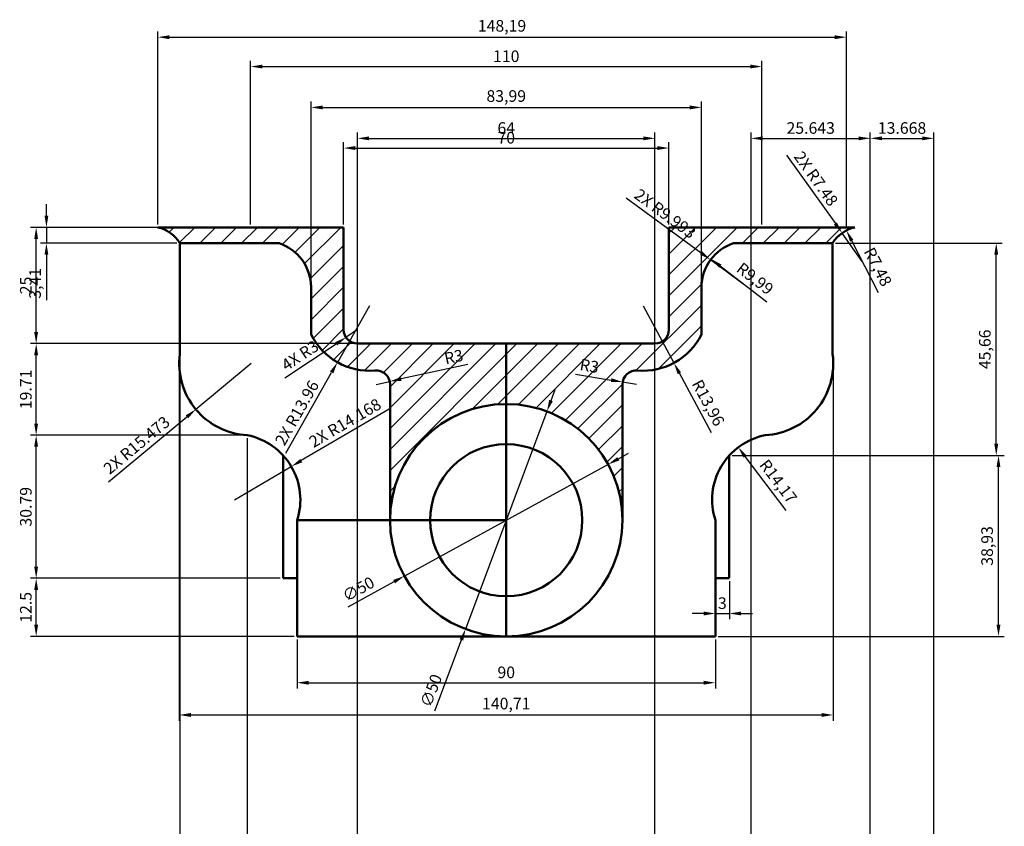
# Model space of a CAD drawing. Units: millimetres. Extents: x 2172 to 2566, y 897 to 1244.
# Tile 2 of 3: x 2172 to 2384, y 1071 to 1244. Entities that reach past the tile are written whole.
import ezdxf

# ---------------------------------------------------------------- set-up
doc = ezdxf.new("R2010")
doc.units = ezdxf.units.MM
for name, color, linetype, lineweight in [('M-DIMS', 2, 'Continuous', 25), ('M-HATC', 8, 'Continuous', 18), ('M-OUTL', 7, 'Continuous', 50)]:
    doc.layers.add(name, color=color, linetype=linetype, lineweight=lineweight)
doc.styles.get("Standard").update_dxf_attribs({"font": 'arial.ttf'})
doc.dimstyles.new('ISO-25', dxfattribs={"dimtxt": 2.5, "dimasz": 2.5, "dimexe": 1.25, "dimexo": 0.625, "dimtad": 1, "dimtxsty": 'Standard', "dimcen": 2.5, "dimadec": 0, "dimazin": 0, "dimtfac": 1, "dimtmove": 0, "dimatfit": 3, "dimfxl": 1, "dimarcsym": 0})

# ---------------------------------------------------------------- blocks, each defined once
blk = doc.blocks.new('*D19')
at = {"layer": 'Defpoints', "color": 0, "transparency": 16777216}
for p in [(2206.43, 1170.23), (2347.14, 1170.23), (2347.14, 1094.59)]:
    blk.add_point(p, dxfattribs=at)
at = {"layer": 'M-DIMS', "color": 0, "lineweight": -2, "transparency": 16777216}
for p, q in [((2206.43, 1169.6), (2206.43, 1093.34)), ((2347.14, 1169.6), (2347.14, 1093.34)), ((2208.93, 1094.59), (2344.64, 1094.59))]:
    blk.add_line(p, q, dxfattribs=at)
at = {"layer": 'M-DIMS', "color": 0, "transparency": 16777216}
for points in [[(2208.93, 1095.01), (2208.93, 1094.17), (2206.43, 1094.59)], [(2344.64, 1095.01), (2344.64, 1094.17), (2347.14, 1094.59)]]:
    blk.add_solid(points, dxfattribs=at)
at = {"layer": 'M-DIMS', "color": 0, "transparency": 16777216, "insert": (2276.79, 1096.72), "char_height": 2.5, "attachment_point": 5}
blk.add_mtext('140,71', dxfattribs=at)
blk = doc.blocks.new('*D20')
at = {"layer": 'Defpoints', "color": 0, "transparency": 16777216}
for p in [(2231.79, 1111.49), (2321.79, 1111.49), (2321.79, 1101.53)]:
    blk.add_point(p, dxfattribs=at)
at = {"layer": 'M-DIMS', "color": 0, "lineweight": -2, "transparency": 16777216}
for p, q in [((2231.79, 1110.86), (2231.79, 1100.28)), ((2321.79, 1110.86), (2321.79, 1100.28)), ((2234.29, 1101.53), (2319.29, 1101.53))]:
    blk.add_line(p, q, dxfattribs=at)
at = {"layer": 'M-DIMS', "color": 0, "transparency": 16777216}
for points in [[(2234.29, 1101.94), (2234.29, 1101.11), (2231.79, 1101.53)], [(2319.29, 1101.94), (2319.29, 1101.11), (2321.79, 1101.53)]]:
    blk.add_solid(points, dxfattribs=at)
at = {"layer": 'M-DIMS', "color": 0, "transparency": 16777216, "insert": (2276.79, 1103.43), "char_height": 2.5, "attachment_point": 5}
blk.add_mtext('90', dxfattribs=at)
blk = doc.blocks.new('*D21')
at = {"layer": 'Defpoints', "color": 0, "transparency": 16777216}
for p in [(2298.71, 1148.5), (2254.86, 1124.48)]:
    blk.add_point(p, dxfattribs=at)
at = {"layer": 'M-DIMS', "color": 0, "lineweight": -2, "transparency": 16777216}
for p, q in [((2300.91, 1149.7), (2303.1, 1150.9)), ((2298.71, 1148.5), (2254.86, 1124.48)), ((2242.77, 1117.85), (2252.67, 1123.27))]:
    blk.add_line(p, q, dxfattribs=at)
at = {"layer": 'M-DIMS', "color": 0, "transparency": 16777216}
for points in [[(2300.71, 1150.07), (2301.11, 1149.33), (2298.71, 1148.5)], [(2252.47, 1123.64), (2252.87, 1122.91), (2254.86, 1124.48)]]:
    blk.add_solid(points, dxfattribs=at)
at = {"layer": 'M-DIMS', "color": 0, "transparency": 16777216, "insert": (2245.13, 1121.39), "char_height": 2.5, "attachment_point": 5, "rotation": 28.7152}
blk.add_mtext('∅50', dxfattribs=at)
blk = doc.blocks.new('*D22')
at = {"layer": 'Defpoints', "color": 0, "transparency": 16777216}
for p in [(2326.7, 1152.17), (2335.26, 1140.88)]:
    blk.add_point(p, dxfattribs=at)
at = {"layer": 'M-DIMS', "color": 0, "lineweight": -2, "transparency": 16777216}
blk.add_line((2337.02, 1138.56), (2328.21, 1150.18), dxfattribs=at)
at = {"layer": 'M-DIMS', "color": 0, "transparency": 16777216}
blk.add_solid([(2328.54, 1150.43), (2327.88, 1149.92), (2326.7, 1152.17)], dxfattribs=at)
at = {"layer": 'M-DIMS', "color": 0, "transparency": 16777216, "insert": (2335.07, 1144.65), "char_height": 2.5, "attachment_point": 5, "rotation": 307.1523}
blk.add_mtext('R14,17', dxfattribs=at)
blk = doc.blocks.new('*D23')
at = {"layer": 'Defpoints', "color": 0, "transparency": 16777216}
for p in [(2306.24, 1182.6), (2312.86, 1170.31)]:
    blk.add_point(p, dxfattribs=at)
at = {"layer": 'M-DIMS', "color": 0, "lineweight": -2, "transparency": 16777216}
for p, q in [((2306.24, 1182.6), (2312.86, 1170.31)), ((2320.96, 1155.28), (2314.04, 1168.11))]:
    blk.add_line(p, q, dxfattribs=at)
at = {"layer": 'M-DIMS', "color": 0, "transparency": 16777216}
blk.add_solid([(2314.41, 1168.31), (2313.68, 1167.91), (2312.86, 1170.31)], dxfattribs=at)
at = {"layer": 'M-DIMS', "color": 0, "transparency": 16777216, "insert": (2319.97, 1161.6), "char_height": 2.5, "attachment_point": 5, "rotation": 298.3069}
blk.add_mtext('R13,96', dxfattribs=at)
blk = doc.blocks.new('*D24')
at = {"layer": 'Defpoints', "color": 0, "transparency": 16777216}
for p in [(2320.87, 1192.69), (2328.77, 1186.58)]:
    blk.add_point(p, dxfattribs=at)
at = {"layer": 'M-DIMS', "color": 0, "lineweight": -2, "transparency": 16777216}
blk.add_line((2332.85, 1183.43), (2322.85, 1191.16), dxfattribs=at)
at = {"layer": 'M-DIMS', "color": 0, "transparency": 16777216}
blk.add_solid([(2323.1, 1191.49), (2322.59, 1190.83), (2320.87, 1192.69)], dxfattribs=at)
at = {"layer": 'M-DIMS', "color": 0, "transparency": 16777216, "insert": (2330.14, 1188.21), "char_height": 2.5, "attachment_point": 5, "rotation": 322.2747}
blk.add_mtext('R9,99', dxfattribs=at)
blk = doc.blocks.new('*D25')
at = {"layer": 'Defpoints', "color": 0, "transparency": 16777216}
for p in [(2349.98, 1198.83), (2353.4, 1192.18)]:
    blk.add_point(p, dxfattribs=at)
at = {"layer": 'M-DIMS', "color": 0, "lineweight": -2, "transparency": 16777216}
blk.add_line((2356.9, 1185.37), (2351.12, 1196.61), dxfattribs=at)
at = {"layer": 'M-DIMS', "color": 0, "transparency": 16777216}
blk.add_solid([(2351.49, 1196.8), (2350.75, 1196.42), (2349.98, 1198.83)], dxfattribs=at)
at = {"layer": 'M-DIMS', "color": 0, "transparency": 16777216, "insert": (2356.48, 1190.85), "char_height": 2.5, "attachment_point": 5, "rotation": 297.2217}
blk.add_mtext('R7,48', dxfattribs=at)
blk = doc.blocks.new('*D26')
at = {"layer": 'Defpoints', "color": 0, "transparency": 16777216}
for p in [(2311.79, 1216.55), (2241.79, 1199.49), (2311.79, 1199.49)]:
    blk.add_point(p, dxfattribs=at)
at = {"layer": 'M-DIMS', "color": 0, "lineweight": -2, "transparency": 16777216}
for p, q in [((2241.79, 1200.11), (2241.79, 1217.8)), ((2244.29, 1216.55), (2309.29, 1216.55)), ((2311.79, 1200.11), (2311.79, 1217.8))]:
    blk.add_line(p, q, dxfattribs=at)
at = {"layer": 'M-DIMS', "color": 0, "transparency": 16777216}
for points in [[(2244.29, 1216.97), (2244.29, 1216.13), (2241.79, 1216.55)], [(2309.29, 1216.97), (2309.29, 1216.13), (2311.79, 1216.55)]]:
    blk.add_solid(points, dxfattribs=at)
at = {"layer": 'M-DIMS', "color": 0, "transparency": 16777216, "insert": (2276.79, 1218.45), "char_height": 2.5, "attachment_point": 5}
blk.add_mtext('70', dxfattribs=at)
blk = doc.blocks.new('*D27')
at = {"layer": 'Defpoints', "color": 0, "transparency": 16777216}
for p in [(2318.78, 1225.29), (2234.79, 1176.47), (2318.78, 1176.47)]:
    blk.add_point(p, dxfattribs=at)
at = {"layer": 'M-DIMS', "color": 0, "lineweight": -2, "transparency": 16777216}
for p, q in [((2234.79, 1177.1), (2234.79, 1226.54)), ((2237.29, 1225.29), (2316.28, 1225.29)), ((2318.78, 1177.1), (2318.78, 1226.54))]:
    blk.add_line(p, q, dxfattribs=at)
at = {"layer": 'M-DIMS', "color": 0, "transparency": 16777216}
for points in [[(2237.29, 1225.71), (2237.29, 1224.87), (2234.79, 1225.29)], [(2316.28, 1225.71), (2316.28, 1224.87), (2318.78, 1225.29)]]:
    blk.add_solid(points, dxfattribs=at)
at = {"layer": 'M-DIMS', "color": 0, "transparency": 16777216, "insert": (2276.79, 1227.42), "char_height": 2.5, "attachment_point": 5}
blk.add_mtext('83,99', dxfattribs=at)
blk = doc.blocks.new('*D28')
at = {"layer": 'Defpoints', "color": 0, "transparency": 16777216}
for p in [(2331.79, 1234.08), (2221.79, 1199.49), (2331.79, 1199.49)]:
    blk.add_point(p, dxfattribs=at)
at = {"layer": 'M-DIMS', "color": 0, "lineweight": -2, "transparency": 16777216}
for p, q in [((2221.79, 1200.11), (2221.79, 1235.33)), ((2331.79, 1200.11), (2331.79, 1235.33)), ((2224.29, 1234.08), (2329.29, 1234.08))]:
    blk.add_line(p, q, dxfattribs=at)
at = {"layer": 'M-DIMS', "color": 0, "transparency": 16777216}
for points in [[(2224.29, 1234.5), (2224.29, 1233.67), (2221.79, 1234.08)], [(2329.29, 1234.5), (2329.29, 1233.67), (2331.79, 1234.08)]]:
    blk.add_solid(points, dxfattribs=at)
at = {"layer": 'M-DIMS', "color": 0, "transparency": 16777216, "insert": (2276.79, 1235.98), "char_height": 2.5, "attachment_point": 5}
blk.add_mtext('110', dxfattribs=at)
blk = doc.blocks.new('*D29')
at = {"layer": 'Defpoints', "color": 0, "transparency": 16777216}
for p in [(2349.98, 1240.4), (2201.79, 1199.49), (2349.98, 1198.83)]:
    blk.add_point(p, dxfattribs=at)
at = {"layer": 'M-DIMS', "color": 0, "lineweight": -2, "transparency": 16777216}
for p, q in [((2201.79, 1200.11), (2201.79, 1241.65)), ((2349.98, 1199.46), (2349.98, 1241.65)), ((2204.29, 1240.4), (2347.48, 1240.4))]:
    blk.add_line(p, q, dxfattribs=at)
at = {"layer": 'M-DIMS', "color": 0, "transparency": 16777216}
for points in [[(2204.29, 1240.81), (2204.29, 1239.98), (2201.79, 1240.4)], [(2347.48, 1240.81), (2347.48, 1239.98), (2349.98, 1240.4)]]:
    blk.add_solid(points, dxfattribs=at)
at = {"layer": 'M-DIMS', "color": 0, "transparency": 16777216, "insert": (2275.88, 1242.52), "char_height": 2.5, "attachment_point": 5}
blk.add_mtext('148,19', dxfattribs=at)
blk = doc.blocks.new('*D30')
at = {"layer": 'Defpoints', "color": 0, "transparency": 16777216}
for p in [(2324.79, 1150.42), (2382.71, 1150.42), (2321.79, 1111.49)]:
    blk.add_point(p, dxfattribs=at)
at = {"layer": 'M-DIMS', "color": 0, "lineweight": -2, "transparency": 16777216}
for p, q in [((2325.41, 1150.42), (2383.96, 1150.42)), ((2382.71, 1113.99), (2382.71, 1147.92)), ((2322.41, 1111.49), (2383.96, 1111.49))]:
    blk.add_line(p, q, dxfattribs=at)
at = {"layer": 'M-DIMS', "color": 0, "transparency": 16777216}
for points in [[(2382.29, 1147.92), (2383.12, 1147.92), (2382.71, 1150.42)], [(2382.29, 1113.99), (2383.12, 1113.99), (2382.71, 1111.49)]]:
    blk.add_solid(points, dxfattribs=at)
at = {"layer": 'M-DIMS', "color": 0, "transparency": 16777216, "insert": (2380.58, 1130.95), "char_height": 2.5, "attachment_point": 5, "rotation": 90}
blk.add_mtext('38,93', dxfattribs=at)
blk = doc.blocks.new('*D31')
at = {"layer": 'Defpoints', "color": 0, "transparency": 16777216}
for p in [(2347.01, 1196.08), (2382.22, 1196.08), (2324.79, 1150.42)]:
    blk.add_point(p, dxfattribs=at)
at = {"layer": 'M-DIMS', "color": 0, "lineweight": -2, "transparency": 16777216}
for p, q in [((2347.64, 1196.08), (2383.47, 1196.08)), ((2382.22, 1152.92), (2382.22, 1193.58)), ((2325.41, 1150.42), (2383.47, 1150.42))]:
    blk.add_line(p, q, dxfattribs=at)
at = {"layer": 'M-DIMS', "color": 0, "transparency": 16777216}
for points in [[(2381.8, 1193.58), (2382.64, 1193.58), (2382.22, 1196.08)], [(2381.8, 1152.92), (2382.64, 1152.92), (2382.22, 1150.42)]]:
    blk.add_solid(points, dxfattribs=at)
at = {"layer": 'M-DIMS', "color": 0, "transparency": 16777216, "insert": (2380.09, 1173.25), "char_height": 2.5, "attachment_point": 5, "rotation": 90}
blk.add_mtext('45,66', dxfattribs=at)
blk = doc.blocks.new('*D32')
at = {"layer": 'Defpoints', "color": 0, "transparency": 16777216}
for p in [(2201.79, 1199.49), (2177.85, 1196.08), (2206.56, 1196.08)]:
    blk.add_point(p, dxfattribs=at)
at = {"layer": 'M-DIMS', "color": 0, "lineweight": -2, "transparency": 16777216}
for p, q in [((2177.85, 1201.99), (2177.85, 1204.49)), ((2201.16, 1199.49), (2176.6, 1199.49)), ((2177.85, 1199.49), (2177.85, 1196.08)), ((2205.94, 1196.08), (2176.6, 1196.08)), ((2177.85, 1193.58), (2177.85, 1183.82))]:
    blk.add_line(p, q, dxfattribs=at)
at = {"layer": 'M-DIMS', "color": 0, "transparency": 16777216}
for points in [[(2177.43, 1201.99), (2178.26, 1201.99), (2177.85, 1199.49)], [(2177.43, 1193.58), (2178.26, 1193.58), (2177.85, 1196.08)]]:
    blk.add_solid(points, dxfattribs=at)
at = {"layer": 'M-DIMS', "color": 0, "transparency": 16777216, "insert": (2175.72, 1187.45), "char_height": 2.5, "attachment_point": 5, "rotation": 90}
blk.add_mtext('3,41', dxfattribs=at)
blk = doc.blocks.new('*D33')
at = {"layer": 'Defpoints', "color": 0, "transparency": 16777216}
for p in [(2321.79, 1123.99), (2324.79, 1123.99), (2324.79, 1116.42)]:
    blk.add_point(p, dxfattribs=at)
at = {"layer": 'M-DIMS', "color": 0, "lineweight": -2, "transparency": 16777216}
for p, q in [((2321.79, 1123.36), (2321.79, 1115.17)), ((2324.79, 1123.36), (2324.79, 1115.17)), ((2319.29, 1116.42), (2316.79, 1116.42)), ((2321.79, 1116.42), (2324.79, 1116.42)), ((2327.29, 1116.42), (2329.79, 1116.42))]:
    blk.add_line(p, q, dxfattribs=at)
at = {"layer": 'M-DIMS', "color": 0, "transparency": 16777216}
for points in [[(2319.29, 1116.84), (2319.29, 1116.01), (2321.79, 1116.42)], [(2327.29, 1116.84), (2327.29, 1116.01), (2324.79, 1116.42)]]:
    blk.add_solid(points, dxfattribs=at)
at = {"layer": 'M-DIMS', "color": 0, "transparency": 16777216, "insert": (2323.29, 1118.32), "char_height": 2.5, "attachment_point": 5}
blk.add_mtext('3', dxfattribs=at)
blk = doc.blocks.new('*D34')
at = {"layer": 'Defpoints', "color": 0, "transparency": 16777216}
for p in [(2248.79, 1165.7), (2251.72, 1166.34)]:
    blk.add_point(p, dxfattribs=at)
at = {"layer": 'M-DIMS', "color": 0, "lineweight": -2, "transparency": 16777216}
for p, q in [((2268.54, 1170.02), (2254.16, 1166.88)), ((2248.79, 1165.7), (2251.72, 1166.34))]:
    blk.add_line(p, q, dxfattribs=at)
at = {"layer": 'M-DIMS', "color": 0, "transparency": 16777216}
blk.add_solid([(2254.07, 1167.29), (2254.25, 1166.47), (2251.72, 1166.34)], dxfattribs=at)
at = {"layer": 'M-DIMS', "color": 0, "transparency": 16777216, "insert": (2265.56, 1171.32), "char_height": 2.5, "attachment_point": 5, "rotation": 12.3382}
blk.add_mtext('R3', dxfattribs=at)
blk = doc.blocks.new('*D35')
at = {"layer": 'Defpoints', "color": 0, "transparency": 16777216}
for p in [(2301.83, 1166.21), (2304.79, 1165.7)]:
    blk.add_point(p, dxfattribs=at)
at = {"layer": 'M-DIMS', "color": 0, "lineweight": -2, "transparency": 16777216}
for p, q in [((2291.7, 1167.94), (2299.37, 1166.63)), ((2304.79, 1165.7), (2301.83, 1166.21))]:
    blk.add_line(p, q, dxfattribs=at)
at = {"layer": 'M-DIMS', "color": 0, "transparency": 16777216}
blk.add_solid([(2299.44, 1167.04), (2299.3, 1166.22), (2301.83, 1166.21)], dxfattribs=at)
at = {"layer": 'M-DIMS', "color": 0, "transparency": 16777216, "insert": (2294.62, 1169.37), "char_height": 2.5, "attachment_point": 5, "rotation": 350.3234}
blk.add_mtext('R3', dxfattribs=at)
blk = doc.blocks.new('*D36')
at = {"layer": 'Defpoints', "color": 0, "transparency": 16777216}
for p in [(2175.64, 1123.99), (2228.79, 1123.99), (2231.79, 1111.49)]:
    blk.add_point(p, dxfattribs=at)
at = {"layer": 'M-DIMS', "color": 0, "lineweight": -2, "transparency": 16777216}
for p, q in [((2228.16, 1123.99), (2174.39, 1123.99)), ((2175.64, 1113.99), (2175.64, 1121.49)), ((2231.16, 1111.49), (2174.39, 1111.49))]:
    blk.add_line(p, q, dxfattribs=at)
at = {"layer": 'M-DIMS', "color": 0, "transparency": 16777216}
for points in [[(2175.22, 1121.49), (2176.05, 1121.49), (2175.64, 1123.99)], [(2175.22, 1113.99), (2176.05, 1113.99), (2175.64, 1111.49)]]:
    blk.add_solid(points, dxfattribs=at)
at = {"layer": 'M-DIMS', "color": 0, "transparency": 16777216, "insert": (2173.74, 1117.74), "char_height": 2.5, "attachment_point": 5, "rotation": 90}
blk.add_mtext('12.5', dxfattribs=at)
blk = doc.blocks.new('*D37')
at = {"layer": 'Defpoints', "color": 0, "transparency": 16777216}
for p in [(2175.64, 1154.78), (2221.06, 1154.78), (2228.79, 1123.99)]:
    blk.add_point(p, dxfattribs=at)
at = {"layer": 'M-DIMS', "color": 0, "lineweight": -2, "transparency": 16777216}
for p, q in [((2220.43, 1154.78), (2174.39, 1154.78)), ((2175.64, 1126.49), (2175.64, 1152.28)), ((2228.16, 1123.99), (2174.39, 1123.99))]:
    blk.add_line(p, q, dxfattribs=at)
at = {"layer": 'M-DIMS', "color": 0, "transparency": 16777216}
for points in [[(2175.22, 1152.28), (2176.05, 1152.28), (2175.64, 1154.78)], [(2175.22, 1126.49), (2176.05, 1126.49), (2175.64, 1123.99)]]:
    blk.add_solid(points, dxfattribs=at)
at = {"layer": 'M-DIMS', "color": 0, "transparency": 16777216, "insert": (2173.74, 1139.38), "char_height": 2.5, "attachment_point": 5, "rotation": 90}
blk.add_mtext('30.79', dxfattribs=at)
blk = doc.blocks.new('*D38')
at = {"layer": 'Defpoints', "color": 0, "transparency": 16777216}
for p in [(2175.64, 1174.49), (2244.79, 1174.49), (2221.06, 1154.78)]:
    blk.add_point(p, dxfattribs=at)
at = {"layer": 'M-DIMS', "color": 0, "lineweight": -2, "transparency": 16777216}
for p, q in [((2244.16, 1174.49), (2174.39, 1174.49)), ((2175.64, 1157.28), (2175.64, 1171.99)), ((2220.43, 1154.78), (2174.39, 1154.78))]:
    blk.add_line(p, q, dxfattribs=at)
at = {"layer": 'M-DIMS', "color": 0, "transparency": 16777216}
for points in [[(2175.22, 1171.99), (2176.05, 1171.99), (2175.64, 1174.49)], [(2175.22, 1157.28), (2176.05, 1157.28), (2175.64, 1154.78)]]:
    blk.add_solid(points, dxfattribs=at)
at = {"layer": 'M-DIMS', "color": 0, "transparency": 16777216, "insert": (2173.74, 1164.63), "char_height": 2.5, "attachment_point": 5, "rotation": 90}
blk.add_mtext('19.71', dxfattribs=at)
blk = doc.blocks.new('*D39')
at = {"layer": 'Defpoints', "color": 0, "transparency": 16777216}
for p in [(2175.64, 1199.49), (2241.79, 1199.49), (2244.79, 1174.49)]:
    blk.add_point(p, dxfattribs=at)
at = {"layer": 'M-DIMS', "color": 0, "lineweight": -2, "transparency": 16777216}
for p, q in [((2241.16, 1199.49), (2174.39, 1199.49)), ((2175.64, 1176.99), (2175.64, 1196.99)), ((2244.16, 1174.49), (2174.39, 1174.49))]:
    blk.add_line(p, q, dxfattribs=at)
at = {"layer": 'M-DIMS', "color": 0, "transparency": 16777216}
for points in [[(2175.22, 1196.99), (2176.05, 1196.99), (2175.64, 1199.49)], [(2175.22, 1176.99), (2176.05, 1176.99), (2175.64, 1174.49)]]:
    blk.add_solid(points, dxfattribs=at)
at = {"layer": 'M-DIMS', "color": 0, "transparency": 16777216, "insert": (2173.74, 1186.99), "char_height": 2.5, "attachment_point": 5, "rotation": 90}
blk.add_mtext('25', dxfattribs=at)
blk = doc.blocks.new('*D40')
at = {"layer": 'Defpoints', "color": 0, "transparency": 16777216}
for p in [(2206.56, 1172.22), (2221.06, 1154.78), (2221.06, 906.81)]:
    blk.add_point(p, dxfattribs=at)
at = {"layer": 'M-DIMS', "color": 0, "lineweight": -2, "transparency": 16777216}
for p, q in [((2206.56, 1171.6), (2206.56, 905.56)), ((2221.06, 1154.15), (2221.06, 905.56)), ((2209.06, 906.81), (2218.56, 906.81))]:
    blk.add_line(p, q, dxfattribs=at)
at = {"layer": 'M-DIMS', "color": 0, "transparency": 16777216}
for points in [[(2209.06, 907.23), (2209.06, 906.4), (2206.56, 906.81)], [(2218.56, 907.23), (2218.56, 906.4), (2221.06, 906.81)]]:
    blk.add_solid(points, dxfattribs=at)
at = {"layer": 'M-DIMS', "color": 0, "transparency": 16777216, "insert": (2213.81, 908.71), "char_height": 2.5, "attachment_point": 5}
blk.add_mtext('14.498', dxfattribs=at)
blk = doc.blocks.new('*D44')
at = {"layer": 'Defpoints', "color": 0, "transparency": 16777216}
for p in [(2355.12, 1218.64), (2329.48, 1046.33), (2355.12, 1035.65)]:
    blk.add_point(p, dxfattribs=at)
at = {"layer": 'M-DIMS', "color": 0, "lineweight": -2, "transparency": 16777216}
for p, q in [((2329.48, 1046.96), (2329.48, 1219.89)), ((2331.98, 1218.64), (2352.62, 1218.64)), ((2355.12, 1036.27), (2355.12, 1219.89))]:
    blk.add_line(p, q, dxfattribs=at)
at = {"layer": 'M-DIMS', "color": 0, "transparency": 16777216}
for points in [[(2331.98, 1219.05), (2331.98, 1218.22), (2329.48, 1218.64)], [(2352.62, 1219.05), (2352.62, 1218.22), (2355.12, 1218.64)]]:
    blk.add_solid(points, dxfattribs=at)
at = {"layer": 'M-DIMS', "color": 0, "transparency": 16777216, "insert": (2342.3, 1220.54), "char_height": 2.5, "attachment_point": 5}
blk.add_mtext('25.643', dxfattribs=at)
blk = doc.blocks.new('*D45')
at = {"layer": 'Defpoints', "color": 0, "transparency": 16777216}
for p in [(2368.79, 1218.64), (2368.79, 1046.33), (2355.12, 1035.65)]:
    blk.add_point(p, dxfattribs=at)
at = {"layer": 'M-DIMS', "color": 0, "lineweight": -2, "transparency": 16777216}
for p, q in [((2355.12, 1036.27), (2355.12, 1219.89)), ((2357.62, 1218.64), (2366.29, 1218.64)), ((2368.79, 1046.96), (2368.79, 1219.89))]:
    blk.add_line(p, q, dxfattribs=at)
at = {"layer": 'M-DIMS', "color": 0, "transparency": 16777216}
for points in [[(2357.62, 1219.05), (2357.62, 1218.22), (2355.12, 1218.64)], [(2366.29, 1219.05), (2366.29, 1218.22), (2368.79, 1218.64)]]:
    blk.add_solid(points, dxfattribs=at)
at = {"layer": 'M-DIMS', "color": 0, "transparency": 16777216, "insert": (2361.95, 1220.54), "char_height": 2.5, "attachment_point": 5}
blk.add_mtext('13.668', dxfattribs=at)
blk = doc.blocks.new('*D54')
at = {"layer": 'Defpoints', "color": 0, "transparency": 16777216}
for p in [(2308.79, 1218.64), (2244.79, 1051.26), (2308.79, 1051.26)]:
    blk.add_point(p, dxfattribs=at)
at = {"layer": 'M-DIMS', "color": 0, "lineweight": -2, "transparency": 16777216}
for p, q in [((2244.79, 1051.88), (2244.79, 1219.89)), ((2247.29, 1218.64), (2306.29, 1218.64)), ((2308.79, 1051.88), (2308.79, 1219.89))]:
    blk.add_line(p, q, dxfattribs=at)
at = {"layer": 'M-DIMS', "color": 0, "transparency": 16777216}
for points in [[(2247.29, 1219.05), (2247.29, 1218.22), (2244.79, 1218.64)], [(2306.29, 1219.05), (2306.29, 1218.22), (2308.79, 1218.64)]]:
    blk.add_solid(points, dxfattribs=at)
at = {"layer": 'M-DIMS', "color": 0, "transparency": 16777216, "insert": (2276.79, 1220.54), "char_height": 2.5, "attachment_point": 5}
blk.add_mtext('64', dxfattribs=at)
blk = doc.blocks.new('*D61')
at = {"layer": 'Defpoints', "color": 0, "transparency": 16777216}
for p in [(2285.55, 1159.9), (2268.03, 1113.07)]:
    blk.add_point(p, dxfattribs=at)
at = {"layer": 'M-DIMS', "color": 0, "lineweight": -2, "transparency": 16777216}
for p, q in [((2286.42, 1162.24), (2287.3, 1164.58)), ((2285.55, 1159.9), (2268.03, 1113.07)), ((2261.45, 1095.49), (2267.15, 1110.73))]:
    blk.add_line(p, q, dxfattribs=at)
at = {"layer": 'M-DIMS', "color": 0, "transparency": 16777216}
for points in [[(2286.03, 1162.39), (2286.81, 1162.1), (2285.55, 1159.9)], [(2266.76, 1110.88), (2267.54, 1110.58), (2268.03, 1113.07)]]:
    blk.add_solid(points, dxfattribs=at)
at = {"layer": 'M-DIMS', "color": 0, "transparency": 16777216, "insert": (2260.92, 1099.71), "char_height": 2.5, "attachment_point": 5, "rotation": 69.487}
blk.add_mtext('∅50', dxfattribs=at)
blk = doc.blocks.new('*D62')
at = {"layer": 'Defpoints', "color": 0, "transparency": 16777216}
for p in [(2221.9, 1170.23), (2210, 1160.34)]:
    blk.add_point(p, dxfattribs=at)
at = {"layer": 'M-DIMS', "color": 0, "lineweight": -2, "transparency": 16777216}
for p, q in [((2221.9, 1170.23), (2210, 1160.34)), ((2191.21, 1144.72), (2208.08, 1158.74))]:
    blk.add_line(p, q, dxfattribs=at)
at = {"layer": 'M-DIMS', "color": 0, "transparency": 16777216}
blk.add_solid([(2207.81, 1159.06), (2208.35, 1158.42), (2210, 1160.34)], dxfattribs=at)
at = {"layer": 'M-DIMS', "color": 0, "transparency": 16777216, "insert": (2197.47, 1152.39), "char_height": 2.5, "attachment_point": 5, "rotation": 39.7235}
blk.add_mtext('2X R15.473', dxfattribs=at)
blk = doc.blocks.new('*D63')
at = {"layer": 'Defpoints', "color": 0, "transparency": 16777216}
for p in [(2230.54, 1148.04), (2218.32, 1140.88)]:
    blk.add_point(p, dxfattribs=at)
at = {"layer": 'M-DIMS', "color": 0, "lineweight": -2, "transparency": 16777216}
for p, q in [((2251.62, 1160.41), (2232.69, 1149.31)), ((2218.32, 1140.88), (2230.54, 1148.04))]:
    blk.add_line(p, q, dxfattribs=at)
at = {"layer": 'M-DIMS', "color": 0, "transparency": 16777216}
blk.add_solid([(2232.48, 1149.67), (2232.9, 1148.95), (2230.54, 1148.04)], dxfattribs=at)
at = {"layer": 'M-DIMS', "color": 0, "transparency": 16777216, "insert": (2242.27, 1157.13), "char_height": 2.5, "attachment_point": 5, "rotation": 30.3976}
blk.add_mtext('2X R14.168', dxfattribs=at)
blk = doc.blocks.new('*D64')
at = {"layer": 'Defpoints', "color": 0, "transparency": 16777216}
for p in [(2247.34, 1182.6), (2240.46, 1170.45)]:
    blk.add_point(p, dxfattribs=at)
at = {"layer": 'M-DIMS', "color": 0, "lineweight": -2, "transparency": 16777216}
for p, q in [((2247.34, 1182.6), (2240.46, 1170.45)), ((2229.37, 1150.89), (2239.22, 1168.28))]:
    blk.add_line(p, q, dxfattribs=at)
at = {"layer": 'M-DIMS', "color": 0, "transparency": 16777216}
blk.add_solid([(2238.86, 1168.49), (2239.59, 1168.07), (2240.46, 1170.45)], dxfattribs=at)
at = {"layer": 'M-DIMS', "color": 0, "transparency": 16777216, "insert": (2232.03, 1159.43), "char_height": 2.5, "attachment_point": 5, "rotation": 60.467}
blk.add_mtext('2X R13.96', dxfattribs=at)
blk = doc.blocks.new('*D65')
at = {"layer": 'Defpoints', "color": 0, "transparency": 16777216}
for p in [(2320.73, 1192.51), (2328.77, 1186.58)]:
    blk.add_point(p, dxfattribs=at)
at = {"layer": 'M-DIMS', "color": 0, "lineweight": -2, "transparency": 16777216}
for p, q in [((2302.62, 1205.85), (2318.72, 1193.99)), ((2328.77, 1186.58), (2320.73, 1192.51))]:
    blk.add_line(p, q, dxfattribs=at)
at = {"layer": 'M-DIMS', "color": 0, "transparency": 16777216}
blk.add_solid([(2318.96, 1194.32), (2318.47, 1193.65), (2320.73, 1192.51)], dxfattribs=at)
at = {"layer": 'M-DIMS', "color": 0, "transparency": 16777216, "insert": (2310.79, 1202.19), "char_height": 2.5, "attachment_point": 5, "rotation": 323.6127}
blk.add_mtext('2X R9.993', dxfattribs=at)
blk = doc.blocks.new('*D66')
at = {"layer": 'Defpoints', "color": 0, "transparency": 16777216}
for p in [(2349.05, 1198.27), (2353.4, 1192.18)]:
    blk.add_point(p, dxfattribs=at)
at = {"layer": 'M-DIMS', "color": 0, "lineweight": -2, "transparency": 16777216}
for p, q in [((2337.11, 1215), (2347.6, 1200.31)), ((2353.4, 1192.18), (2349.05, 1198.27))]:
    blk.add_line(p, q, dxfattribs=at)
at = {"layer": 'M-DIMS', "color": 0, "transparency": 16777216}
blk.add_solid([(2347.94, 1200.55), (2347.26, 1200.06), (2349.05, 1198.27)], dxfattribs=at)
at = {"layer": 'M-DIMS', "color": 0, "transparency": 16777216, "insert": (2343.18, 1209.78), "char_height": 2.5, "attachment_point": 5, "rotation": 305.5171}
blk.add_mtext('2X R7.48', dxfattribs=at)
blk = doc.blocks.new('*D67')
at = {"layer": 'Defpoints', "color": 0, "transparency": 16777216}
for p in [(2244.79, 1177.49), (2242.29, 1175.83)]:
    blk.add_point(p, dxfattribs=at)
at = {"layer": 'M-DIMS', "color": 0, "lineweight": -2, "transparency": 16777216}
for p, q in [((2244.79, 1177.49), (2242.29, 1175.83)), ((2229.17, 1167.1), (2240.21, 1174.44))]:
    blk.add_line(p, q, dxfattribs=at)
at = {"layer": 'M-DIMS', "color": 0, "transparency": 16777216}
blk.add_solid([(2239.98, 1174.79), (2240.44, 1174.09), (2242.29, 1175.83)], dxfattribs=at)
at = {"layer": 'M-DIMS', "color": 0, "transparency": 16777216, "insert": (2232.6, 1171.66), "char_height": 2.5, "attachment_point": 5, "rotation": 33.6354}
blk.add_mtext('4X R3', dxfattribs=at)

msp = doc.modelspace()

# ---------------------------------------------------------------- hatches: boundary and pattern name
at = {"layer": 'M-HATC'}
h = msp.add_hatch(dxfattribs=at)
h.set_pattern_fill('ANSI31', color=256)
h.paths.add_polyline_path([(2241.7875, 1199.4872), (2201.7875, 1199.4872, -0.20420698), (2206.5611, 1196.08), (2227.8919, 1196.08, -0.32106205), (2234.7936, 1186.7135), (2234.7936, 1176.4744, 0.30991376), (2248.5309, 1168.6924, -0.43952546), (2251.7875, 1165.7034), (2251.7875, 1136.4872, -0.41421356), (2276.7875, 1161.4872), (2276.7875, 1174.4872), (2244.7875, 1174.4872, -0.41421356), (2241.7875, 1177.4872)])
h.paths.add_polyline_path([(2351.7875, 1199.4872), (2311.7875, 1199.4872), (2311.7875, 1177.4872, -0.41421356), (2308.7875, 1174.4872), (2276.7875, 1174.4872), (2276.7875, 1161.4872, -0.41421356), (2301.7875, 1136.4872), (2301.7875, 1165.7034, -0.43952546), (2305.0442, 1168.6924, 0.30991376), (2318.7815, 1176.4744), (2318.7815, 1186.7135, -0.32106205), (2325.6832, 1196.08), (2347.014, 1196.08, -0.20420698)])
h.paths.add_polyline_path([(2263.264, 1168.1577), (2268.8466, 1169.3788), (2267.7457, 1174.4115), (2262.1632, 1173.1904)], flags=24)
h.paths.add_polyline_path([(2291.3075, 1167.2961), (2296.9408, 1166.3356), (2297.8067, 1171.414), (2292.1735, 1172.3746)], flags=24)

# ---------------------------------------------------------------- linework, layer by layer
at = {"layer": 'M-OUTL'}
for p, q in [((2241.7875, 1199.4872), (2201.7875, 1199.4872)), ((2241.7875, 1177.4872), (2241.7875, 1199.4872)), ((2311.7875, 1199.4872), (2311.7875, 1177.4872)), ((2311.7875, 1199.4872), (2351.7875, 1199.4872)), ((2206.5611, 1172.2234), (2206.5611, 1196.08)), ((2206.5611, 1196.08), (2227.8919, 1196.08)), ((2347.014, 1196.08), (2325.6832, 1196.08)), ((2347.014, 1172.2234), (2347.014, 1196.08)), ((2234.7936, 1186.7135), (2234.7936, 1176.4744)), ((2318.7815, 1186.7135), (2318.7815, 1176.4744)), ((2308.7875, 1174.4872), (2244.7875, 1174.4872)), ((2276.7875, 1174.4872), (2276.7875, 1111.4872)), ((2251.7875, 1136.4872), (2251.7875, 1165.7034)), ((2301.7875, 1136.4872), (2301.7875, 1165.7034)), ((2228.7875, 1123.9872), (2228.7875, 1150.4189)), ((2324.7875, 1123.9872), (2324.7875, 1150.4189)), ((2231.7875, 1111.4872), (2231.7875, 1136.4872)), ((2231.7875, 1136.4872), (2276.7875, 1136.4872)), ((2321.7875, 1111.4872), (2321.7875, 1136.4872)), ((2231.7875, 1123.9872), (2228.7875, 1123.9872)), ((2321.7875, 1111.4872), (2321.7875, 1123.9872)), ((2321.7875, 1123.9872), (2324.7875, 1123.9872)), ((2276.7875, 1111.4872), (2231.7875, 1111.4872)), ((2276.7875, 1111.4872), (2321.7875, 1111.4872))]:
    msp.add_line(p, q, dxfattribs=at)
for radius in [25, 16.3696]:
    msp.add_circle((2276.7875, 1136.4872), radius, dxfattribs=at)
for centre, radius, start, end in [((2200.177, 1192.1833), 7.4794, 31.39905, 77.565111), ((2353.3981, 1192.1833), 7.4794, 102.434889, 148.60095), ((2224.8012, 1186.5766), 9.9934, 0.785155, 71.984568), ((2328.7739, 1186.5766), 9.9934, 108.015432, 179.214845), ((2247.3369, 1182.6006), 13.9594, 206.031134, 274.906846), ((2244.7875, 1177.4872), 3, 180, 270), ((2306.2382, 1182.6006), 13.9594, 265.093154, 333.968866), ((2308.7875, 1177.4872), 3, 270, 0), ((2221.9043, 1170.2251), 15.4728, 172.579338, 266.868139), ((2331.6708, 1170.2251), 15.4728, 273.131861, 7.420662), ((2248.7875, 1165.7034), 3, 0, 94.906846), ((2304.7875, 1165.7034), 3, 85.093154, 180), ((2218.3158, 1140.8751), 14.1684, 341.958905, 78.836174), ((2335.2593, 1140.8751), 14.1684, 101.163826, 198.041095)]:
    msp.add_arc(centre, radius, start, end, dxfattribs=at)

# ---------------------------------------------------------------- dimensions: what is measured, and where the dimension line sits
at = {"layer": 'M-DIMS'}
for base, p1, p2, override, picture, middle in [((2349.9768, 1240.3952), (2201.7875, 1199.4872), (2349.9768, 1198.8342), {"dimclrd": 0, "dimclre": 0, "dimclrt": 0}, '*D29', (2275.8822, 1242.5226)), ((2331.7875, 1234.0825), (2221.7875, 1199.4872), (2331.7875, 1199.4872), {"dimclrd": 0, "dimclre": 0, "dimclrt": 0}, '*D28', (2276.7875, 1235.9839)), ((2318.7815, 1225.2914), (2234.7936, 1176.4744), (2318.7815, 1176.4744), {"dimclrd": 0, "dimclre": 0, "dimclrt": 0}, '*D27', (2276.7875, 1227.4188)), ((2308.7875, 1218.6372), (2244.7875, 1051.2565), (2308.7875, 1051.2565), {"dimdec": 0, "dimlfac": 1, "dimrnd": 0, "dimzin": 0, "dimdsep": 46, "dimlunit": 2}, '*D54', (2276.7875, 1220.5386)), ((2355.12, 1218.6372), (2329.4768, 1046.3302), (2355.12, 1035.65), {"dimdec": 3, "dimlfac": 1, "dimrnd": 0, "dimzin": 0, "dimdsep": 46, "dimlunit": 2}, '*D44', (2342.2984, 1220.5395)), ((2368.78755, 1218.63717), (2355.12001, 1035.64997), (2368.78755, 1046.33023), {"dimdec": 3, "dimlfac": 1, "dimrnd": 0, "dimzin": 0, "dimdsep": 46, "dimlunit": 2}, '*D45', (2361.95378, 1220.53946)), ((2311.7875, 1216.5507), (2241.7875, 1199.4872), (2311.7875, 1199.4872), {"dimclrd": 0, "dimclre": 0, "dimclrt": 0}, '*D26', (2276.7875, 1218.4521)), ((2221.059, 906.8126), (2206.5611, 1172.2234), (2221.059, 1154.7754), {"dimdec": 3, "dimlfac": 1, "dimrnd": 0, "dimzin": 0, "dimdsep": 46, "dimlunit": 2}, '*D40', (2213.81, 908.714)), ((2347.1436, 1094.5885), (2206.4315, 1170.2251), (2347.1436, 1170.2251), {"dimclrd": 0, "dimclre": 0, "dimclrt": 0}, '*D19', (2276.7875, 1096.7158)), ((2324.7875, 1116.422), (2321.7875, 1123.9872), (2324.7875, 1123.9872), {"dimclrd": 0, "dimclre": 0, "dimclrt": 0}, '*D33', (2323.2875, 1118.3243)), ((2321.7875, 1101.527), (2231.7875, 1111.4872), (2321.7875, 1111.4872), {"dimclrd": 0, "dimclre": 0, "dimclrt": 0}, '*D20', (2276.7875, 1103.4284))]:
    dim = msp.add_linear_dim(base=base, p1=p1, p2=p2, dimstyle='ISO-25', override=override, dxfattribs=at)
    dim.commit()
    dim.dimension.update_dxf_attribs({"geometry": picture, "text_midpoint": middle})
for center, mpoint, text, override, picture, middle in [((2353.3981, 1192.1833), (2349.053, 1198.271), '2X <>', {"dimdec": 2, "dimlfac": 1, "dimrnd": 0, "dimzin": 0, "dimdsep": 46, "dimlunit": 2}, '*D66', (2343.1773, 1209.7762)), ((2328.7739, 1186.5766), (2320.729, 1192.505), '2X <>', {"dimdec": 3, "dimlfac": 1, "dimrnd": 0, "dimzin": 0, "dimdsep": 46, "dimlunit": 2}, '*D65', (2310.7911, 1202.1914)), ((2247.3369, 1182.6006), (2240.456, 1170.455), '2X <>', {"dimdec": 2, "dimlfac": 1, "dimrnd": 0, "dimzin": 0, "dimdsep": 46, "dimlunit": 2}, '*D64', (2232.0252, 1159.4329)), ((2244.7875, 1177.4872), (2242.2898, 1175.8255), '4X <>', {"dimdec": 0, "dimlfac": 1, "dimrnd": 0, "dimzin": 0, "dimdsep": 46, "dimlunit": 2}, '*D67', (2232.5966, 1171.6614)), ((2221.9043, 1170.2251), (2210.0036, 1160.3367), '2X <>', {"dimdec": 3, "dimlfac": 1, "dimrnd": 0, "dimzin": 0, "dimdsep": 46, "dimlunit": 2}, '*D62', (2197.4679, 1152.3939)), ((2218.3158, 1140.8751), (2230.5365, 1148.0443), '2X <>', {"dimdec": 3, "dimlfac": 1, "dimrnd": 0, "dimzin": 0, "dimdsep": 46, "dimlunit": 2}, '*D63', (2242.2711, 1157.1328))]:
    dim = msp.add_radius_dim(center=center, mpoint=mpoint, text=text, dimstyle='ISO-25', override=override, dxfattribs=at)
    dim.commit()
    dim.dimension.update_dxf_attribs({"geometry": picture, "text_midpoint": middle})
for base, p1, p2, override, picture, middle in [((2177.848, 1196.08), (2201.7875, 1199.4872), (2206.5611, 1196.08), {"dimclrd": 0, "dimclre": 0, "dimclrt": 0}, '*D32', (2175.7206, 1187.4502)), ((2175.6375, 1199.4872), (2244.7875, 1174.4872), (2241.7875, 1199.4872), {"dimdec": 0, "dimlfac": 1, "dimrnd": 0, "dimzin": 0, "dimdsep": 46, "dimlunit": 2}, '*D39', (2173.7361, 1186.9872)), ((2382.2203, 1196.08), (2324.7875, 1150.4189), (2347.014, 1196.08), {"dimclrd": 0, "dimclre": 0, "dimclrt": 0}, '*D31', (2380.0929, 1173.2495)), ((2175.6375, 1174.4872), (2221.059, 1154.7754), (2244.7875, 1174.4872), {"dimdec": 2, "dimlfac": 1, "dimrnd": 0, "dimzin": 0, "dimdsep": 46, "dimlunit": 2}, '*D38', (2173.7361, 1164.6313)), ((2175.6375, 1154.7754), (2228.7875, 1123.9872), (2221.059, 1154.7754), {"dimdec": 2, "dimlfac": 1, "dimrnd": 0, "dimzin": 0, "dimdsep": 46, "dimlunit": 2}, '*D37', (2173.7353, 1139.3813)), ((2382.7063, 1150.4189), (2321.7875, 1111.4872), (2324.7875, 1150.4189), {"dimclrd": 0, "dimclre": 0, "dimclrt": 0}, '*D30', (2380.579, 1130.9531)), ((2175.6375, 1123.9872), (2231.7875, 1111.4872), (2228.7875, 1123.9872), {"dimdec": 1, "dimlfac": 1, "dimrnd": 0, "dimzin": 0, "dimdsep": 46, "dimlunit": 2}, '*D36', (2173.7361, 1117.7372))]:
    dim = msp.add_linear_dim(base=base, p1=p1, p2=p2, angle=90, dimstyle='ISO-25', override=override, dxfattribs=at)
    dim.commit()
    dim.dimension.update_dxf_attribs({"geometry": picture, "text_midpoint": middle})
for center, mpoint, picture, middle in [((2353.3981, 1192.1833), (2349.9768, 1198.8342), '*D25', (2354.5835, 1189.8789)), ((2328.7739, 1186.5766), (2320.8696, 1192.6913), '*D24', (2328.8351, 1186.5292)), ((2248.7875, 1165.7034), (2251.7183, 1166.3444), '*D34', (2265.9632, 1169.4603)), ((2335.2593, 1140.8751), (2326.7025, 1152.1678), '*D22', (2333.3696, 1143.369))]:
    dim = msp.add_radius_dim(center=center, mpoint=mpoint, dimstyle='ISO-25', override={"dimclrd": 0, "dimclre": 0, "dimclrt": 0}, dxfattribs=at)
    dim.commit()
    dim.dimension.update_dxf_attribs({"geometry": picture, "text_midpoint": middle, "dimtype": 164})
for center, mpoint, picture, middle in [((2306.2382, 1182.6006), (2312.8577, 1170.3105), '*D23', (2319.9651, 1161.6008)), ((2304.7875, 1165.7034), (2301.8302, 1166.2077), '*D35', (2294.618, 1169.3672))]:
    dim = msp.add_radius_dim(center=center, mpoint=mpoint, dimstyle='ISO-25', override={"dimclrd": 0, "dimclre": 0, "dimclrt": 0}, dxfattribs=at)
    dim.commit()
    dim.dimension.update_dxf_attribs({"geometry": picture, "text_midpoint": middle})
for p1, p2, override, picture, middle in [((2285.548, 1159.902), (2268.0271, 1113.0723), {"dimdec": 0, "dimlfac": 1, "dimrnd": 0, "dimzin": 0, "dimdsep": 46, "dimlunit": 2}, '*D61', (2262.7708, 1099.0235)), ((2298.713, 1148.4986), (2254.8621, 1124.4758), {"dimclrd": 0, "dimclre": 0, "dimclrt": 0}, '*D21', (2246.0819, 1119.6658))]:
    dim = msp.add_diameter_dim_2p(p1=p1, p2=p2, dimstyle='ISO-25', override=override, dxfattribs=at)
    dim.commit()
    dim.dimension.update_dxf_attribs({"geometry": picture, "text_midpoint": middle, "dimtype": 163})

doc.saveas('drawing.dxf')
